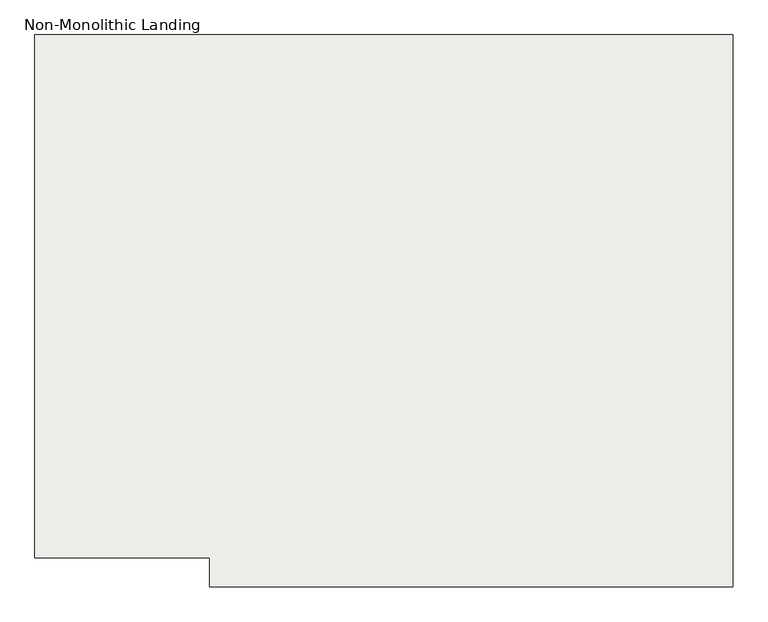
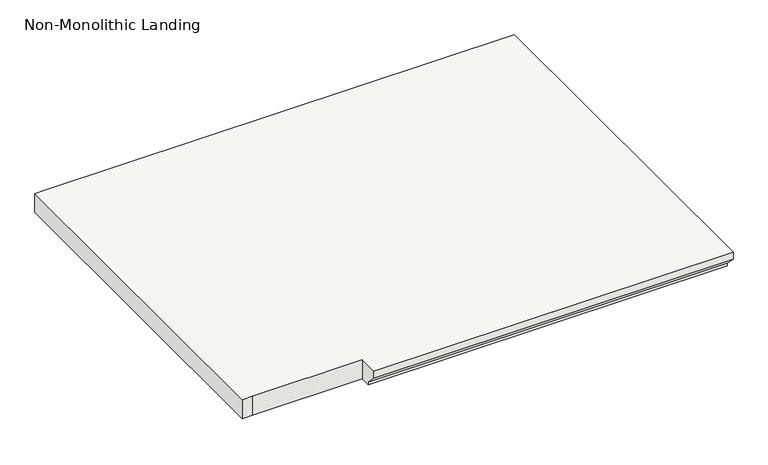
"""IFC4 building model written with IfcOpenShell, lengths in millimetres: slab geometry, Non-Monolithic Landing."""

from ifc_helpers import new_model, si_unit, origin, place, context, project, spatial, faceted_brep, source, transform, mapped, element, save


def non_monolithic_landing_ab58be02(model_context):
    return source(origin(), model_context, "Body", "Brep", [
        faceted_brep([(9871.2423568, -8140.7746824, 5451.3078947), (9871.2423568, -8140.7746824, 5470.3578947), (8956.8423568, -8140.7746824, 5470.3578947), (8956.8423568, -8140.7746824, 5451.3078947), (9871.2423568, -8115.3746824, 5425.9078947), (8956.8423568, -8115.3746824, 5425.9078947), (9871.2423568, -7175.5746824, 5470.3578947), (8676.6463344, -7175.5746824, 5470.3578947), (8651.2463344, -7175.5746824, 5470.3578947), (8651.2463344, -8089.9746824, 5470.3578947), (8676.6463344, -8089.9746824, 5470.3578947), (8956.8423568, -8089.9746824, 5470.3578947), (9871.2423568, -8115.3746824, 5419.5578947), (8956.8423568, -8115.3746824, 5419.5578947), (8956.8423568, -8089.9746824, 5419.5578947), (8676.6463344, -8089.9746824, 5419.5578947), (8651.2463344, -8089.9746824, 5419.5578947), (8651.2463344, -7175.5746824, 5419.5578947), (8676.6463344, -7175.5746824, 5419.5578947), (9871.2423568, -7175.5746824, 5419.5578947)], [[[0, 1, 2, 3]], [[4, 0, 3, 5]], [[6, 7, 8, 9, 10, 11, 2, 1]], [[12, 13, 14, 15, 16, 17, 18, 19]], [[13, 12, 4, 5]], [[6, 1, 0, 4, 12, 19]], [[7, 6, 19, 18]], [[8, 7, 18, 17]], [[9, 8, 17, 16]], [[10, 9, 16, 15]], [[11, 10, 15, 14]], [[2, 11, 14, 13, 5, 3]]]),
    ])


if __name__ == "__main__":
    model = new_model("IFC4")
    model_context = context("Model", 3, world=origin())
    ifc_project = project(units=[si_unit("LENGTHUNIT", "METRE", prefix="MILLI")], contexts=[model_context])
    site = spatial("IfcSite", under=ifc_project)
    building = spatial("IfcBuilding", under=site)
    placement = place(None, origin())
    non_monolithic_landing_shape = non_monolithic_landing_ab58be02(model_context)
    element("IfcSlab", 1, ObjectType="Non-Monolithic Landing", at=placement, inside=building, context=model_context, shape_type="MappedRepresentation", body=[
        mapped(non_monolithic_landing_shape, transform((0.0, 0.0, 0.0), x_axis=(1.0, 0.0, 0.0), y_axis=(0.0, 1.0, 0.0), z_axis=(0.0, 0.0, 1.0))),
    ])
    save(model, "model.ifc")

# Revit data of these elements
# Element 1 (IfcSlab, "Non-Monolithic Landing")
#   Materials on its faces: "MARBLE STAIRS 6\""
# Materials
#   "MARBLE STAIRS 6\"": class "Generic", colour RGB 120 120 120, transparency 0, Cost = 0
